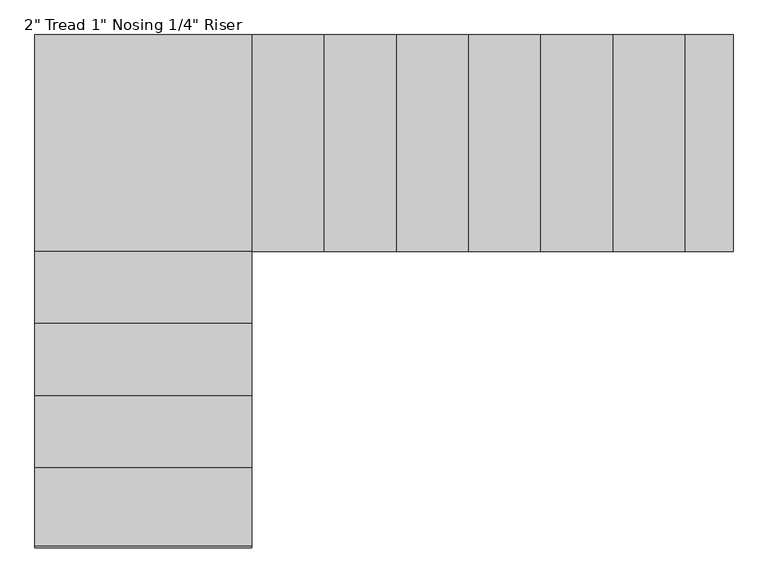
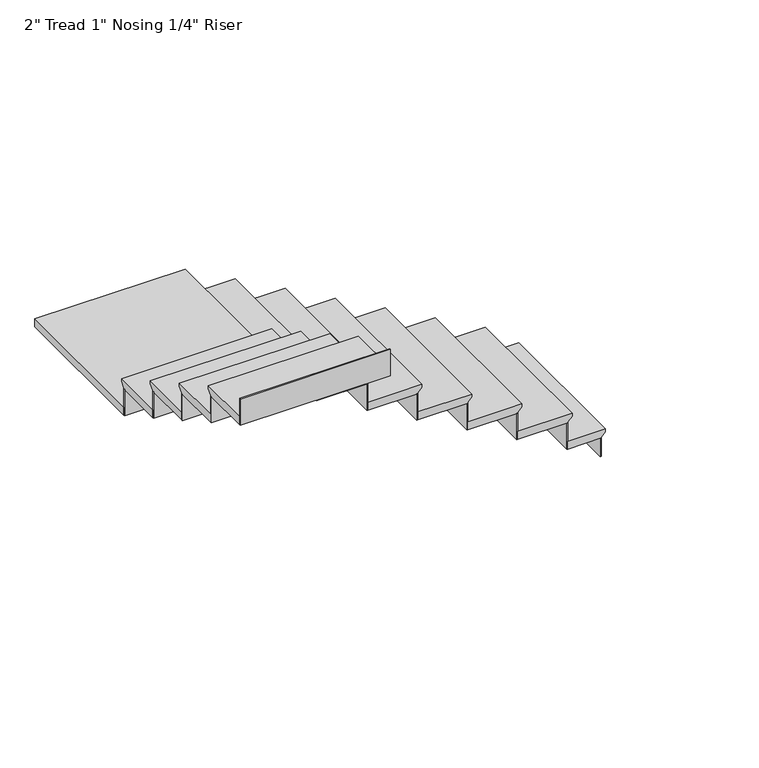
"""IFC4 building model written with IfcOpenShell, lengths in millimetres: stair flight geometry."""

from ifc_helpers import new_model, si_unit, origin, place, context, project, spatial, faceted_brep, source, transform, mapped, element, save


def stair_flight_cf719367(model_context):
    return source(origin(), model_context, "Body", "Brep", [
        faceted_brep([(-442.4415084, 5282.3381995, 3198.2833333), (-442.4415084, 5282.3381995, 3217.3333333), (-442.4415084, 4368.3146777, 3217.3333333), (-442.4415084, 4368.3146777, 3198.2833333), (-467.8415084, 5282.3381995, 3172.8833333), (-467.8415084, 4368.3146777, 3172.8833333), (-671.0415084, 5282.3381995, 3217.3333333), (-671.0415084, 4368.3146777, 3217.3333333), (-467.8415084, 4368.3146777, 3166.5333333), (-671.0415084, 4368.3146777, 3166.5333333), (-671.0415084, 5282.3381995, 3166.5333333), (-467.8415084, 5282.3381995, 3166.5333333)], [[[0, 1, 2, 3]], [[4, 0, 3, 5]], [[2, 1, 6, 7]], [[8, 9, 10, 11]], [[2, 7, 9, 8, 5, 3]], [[8, 11, 4, 5]], [[6, 1, 0, 4, 11, 10]], [[7, 6, 10, 9]]]),
        faceted_brep([(-467.8415084, 5282.3381995, 3166.5333333), (-467.8415084, 5282.3381995, 3048.0), (-474.1915084, 5282.3381995, 3048.0), (-474.1915084, 5282.3381995, 3166.5333333), (-467.8415084, 4368.3146777, 3166.5333333), (-474.1915084, 4368.3146777, 3166.5333333), (-474.1915084, 4368.3146777, 3048.0), (-467.8415084, 4368.3146777, 3048.0)], [[[0, 1, 2, 3]], [[4, 5, 6, 7]], [[1, 0, 4, 7]], [[2, 1, 7, 6]], [[3, 2, 6, 5]], [[0, 3, 5, 4]]]),
        faceted_brep([(-671.0415084, 5282.3381995, 3335.8666667), (-671.0415084, 5282.3381995, 3166.5333333), (-677.3915084, 5282.3381995, 3166.5333333), (-677.3915084, 5282.3381995, 3335.8666667), (-671.0415084, 4368.3146777, 3335.8666667), (-677.3915084, 4368.3146777, 3335.8666667), (-677.3915084, 4368.3146777, 3166.5333333), (-671.0415084, 4368.3146777, 3166.5333333)], [[[0, 1, 2, 3]], [[4, 5, 6, 7]], [[1, 0, 4, 7]], [[2, 1, 7, 6]], [[3, 2, 6, 5]], [[0, 3, 5, 4]]]),
        faceted_brep([(-645.6415084, 4368.3146777, 3386.6666667), (-645.6415084, 5282.3381995, 3386.6666667), (-975.8415084, 5282.3381995, 3386.6666667), (-975.8415084, 4368.3146777, 3386.6666667), (-671.0415084, 4368.3146777, 3335.8666667), (-975.8415084, 4368.3146777, 3335.8666667), (-975.8415084, 5282.3381995, 3335.8666667), (-671.0415084, 5282.3381995, 3335.8666667), (-671.0415084, 4368.3146777, 3342.2166667), (-645.6415084, 4368.3146777, 3367.6166667), (-671.0415084, 5282.3381995, 3342.2166667), (-645.6415084, 5282.3381995, 3367.6166667)], [[[0, 1, 2, 3]], [[4, 5, 6, 7]], [[0, 3, 5, 4, 8, 9]], [[4, 7, 10, 8]], [[2, 1, 11, 10, 7, 6]], [[3, 2, 6, 5]], [[11, 1, 0, 9]], [[10, 11, 9, 8]]]),
        faceted_brep([(-975.8415084, 5282.3381995, 3505.2), (-975.8415084, 5282.3381995, 3335.8666667), (-982.1915084, 5282.3381995, 3335.8666667), (-982.1915084, 5282.3381995, 3505.2), (-975.8415084, 4368.3146777, 3505.2), (-982.1915084, 4368.3146777, 3505.2), (-982.1915084, 4368.3146777, 3335.8666667), (-975.8415084, 4368.3146777, 3335.8666667)], [[[0, 1, 2, 3]], [[4, 5, 6, 7]], [[1, 0, 4, 7]], [[2, 1, 7, 6]], [[3, 2, 6, 5]], [[0, 3, 5, 4]]]),
        faceted_brep([(-950.4415084, 4368.3146777, 3556.0), (-950.4415084, 5282.3381995, 3556.0), (-1280.6415084, 5282.3381995, 3556.0), (-1280.6415084, 4368.3146777, 3556.0), (-975.8415084, 4368.3146777, 3505.2), (-1280.6415084, 4368.3146777, 3505.2), (-1280.6415084, 5282.3381995, 3505.2), (-975.8415084, 5282.3381995, 3505.2), (-975.8415084, 4368.3146777, 3511.55), (-950.4415084, 4368.3146777, 3536.95), (-975.8415084, 5282.3381995, 3511.55), (-950.4415084, 5282.3381995, 3536.95)], [[[0, 1, 2, 3]], [[4, 5, 6, 7]], [[0, 3, 5, 4, 8, 9]], [[4, 7, 10, 8]], [[2, 1, 11, 10, 7, 6]], [[3, 2, 6, 5]], [[11, 1, 0, 9]], [[10, 11, 9, 8]]]),
        faceted_brep([(-1280.6415084, 5282.3381995, 3674.5333333), (-1280.6415084, 5282.3381995, 3505.2), (-1286.9915084, 5282.3381995, 3505.2), (-1286.9915084, 5282.3381995, 3674.5333333), (-1280.6415084, 4368.3146777, 3674.5333333), (-1286.9915084, 4368.3146777, 3674.5333333), (-1286.9915084, 4368.3146777, 3505.2), (-1280.6415084, 4368.3146777, 3505.2)], [[[0, 1, 2, 3]], [[4, 5, 6, 7]], [[1, 0, 4, 7]], [[2, 1, 7, 6]], [[3, 2, 6, 5]], [[0, 3, 5, 4]]]),
        faceted_brep([(-1255.2415084, 4368.3146777, 3725.3333333), (-1255.2415084, 5282.3381995, 3725.3333333), (-1585.4415084, 5282.3381995, 3725.3333333), (-1585.4415084, 4368.3146777, 3725.3333333), (-1280.6415084, 4368.3146777, 3674.5333333), (-1585.4415084, 4368.3146777, 3674.5333333), (-1585.4415084, 5282.3381995, 3674.5333333), (-1280.6415084, 5282.3381995, 3674.5333333), (-1280.6415084, 4368.3146777, 3680.8833333), (-1255.2415084, 4368.3146777, 3706.2833333), (-1280.6415084, 5282.3381995, 3680.8833333), (-1255.2415084, 5282.3381995, 3706.2833333)], [[[0, 1, 2, 3]], [[4, 5, 6, 7]], [[0, 3, 5, 4, 8, 9]], [[4, 7, 10, 8]], [[2, 1, 11, 10, 7, 6]], [[3, 2, 6, 5]], [[11, 1, 0, 9]], [[10, 11, 9, 8]]]),
        faceted_brep([(-1585.4415084, 5282.3381995, 3843.8666667), (-1585.4415084, 5282.3381995, 3674.5333333), (-1591.7915084, 5282.3381995, 3674.5333333), (-1591.7915084, 5282.3381995, 3843.8666667), (-1585.4415084, 4368.3146777, 3843.8666667), (-1591.7915084, 4368.3146777, 3843.8666667), (-1591.7915084, 4368.3146777, 3674.5333333), (-1585.4415084, 4368.3146777, 3674.5333333)], [[[0, 1, 2, 3]], [[4, 5, 6, 7]], [[1, 0, 4, 7]], [[2, 1, 7, 6]], [[3, 2, 6, 5]], [[0, 3, 5, 4]]]),
        faceted_brep([(-1560.0415084, 4368.3146777, 3894.6666667), (-1560.0415084, 5282.3381995, 3894.6666667), (-1890.2415084, 5282.3381995, 3894.6666667), (-1890.2415084, 4368.3146777, 3894.6666667), (-1585.4415084, 4368.3146777, 3843.8666667), (-1890.2415084, 4368.3146777, 3843.8666667), (-1890.2415084, 5282.3381995, 3843.8666667), (-1585.4415084, 5282.3381995, 3843.8666667), (-1585.4415084, 4368.3146777, 3850.2166667), (-1560.0415084, 4368.3146777, 3875.6166667), (-1585.4415084, 5282.3381995, 3850.2166667), (-1560.0415084, 5282.3381995, 3875.6166667)], [[[0, 1, 2, 3]], [[4, 5, 6, 7]], [[0, 3, 5, 4, 8, 9]], [[4, 7, 10, 8]], [[2, 1, 11, 10, 7, 6]], [[3, 2, 6, 5]], [[11, 1, 0, 9]], [[10, 11, 9, 8]]]),
        faceted_brep([(-1890.2415084, 5282.3381995, 4013.2), (-1890.2415084, 5282.3381995, 3843.8666667), (-1896.5915084, 5282.3381995, 3843.8666667), (-1896.5915084, 5282.3381995, 4013.2), (-1890.2415084, 4368.3146777, 4013.2), (-1896.5915084, 4368.3146777, 4013.2), (-1896.5915084, 4368.3146777, 3843.8666667), (-1890.2415084, 4368.3146777, 3843.8666667)], [[[0, 1, 2, 3]], [[4, 5, 6, 7]], [[1, 0, 4, 7]], [[2, 1, 7, 6]], [[3, 2, 6, 5]], [[0, 3, 5, 4]]]),
        faceted_brep([(-1864.8415084, 4368.3146777, 4064.0), (-1864.8415084, 5282.3381995, 4064.0), (-2195.0415084, 5282.3381995, 4064.0), (-2195.0415084, 4368.3146777, 4064.0), (-1890.2415084, 4368.3146777, 4013.2), (-2195.0415084, 4368.3146777, 4013.2), (-2195.0415084, 5282.3381995, 4013.2), (-1890.2415084, 5282.3381995, 4013.2), (-1890.2415084, 4368.3146777, 4019.55), (-1864.8415084, 4368.3146777, 4044.95), (-1890.2415084, 5282.3381995, 4019.55), (-1864.8415084, 5282.3381995, 4044.95)], [[[0, 1, 2, 3]], [[4, 5, 6, 7]], [[0, 3, 5, 4, 8, 9]], [[4, 7, 10, 8]], [[2, 1, 11, 10, 7, 6]], [[3, 2, 6, 5]], [[11, 1, 0, 9]], [[10, 11, 9, 8]]]),
        faceted_brep([(-2195.0415084, 5282.3381995, 4182.5333333), (-2195.0415084, 5282.3381995, 4013.2), (-2201.3915084, 5282.3381995, 4013.2), (-2201.3915084, 5282.3381995, 4182.5333333), (-2195.0415084, 4368.3146777, 4182.5333333), (-2201.3915084, 4368.3146777, 4182.5333333), (-2201.3915084, 4368.3146777, 4013.2), (-2195.0415084, 4368.3146777, 4013.2)], [[[0, 1, 2, 3]], [[4, 5, 6, 7]], [[1, 0, 4, 7]], [[2, 1, 7, 6]], [[3, 2, 6, 5]], [[0, 3, 5, 4]]]),
        faceted_brep([(-2169.6415084, 4368.3146777, 4233.3333333), (-2169.6415084, 5282.3381995, 4233.3333333), (-2499.8415084, 5282.3381995, 4233.3333333), (-2499.8415084, 4368.3146777, 4233.3333333), (-2195.0415084, 4368.3146777, 4182.5333333), (-2499.8415084, 4368.3146777, 4182.5333333), (-2499.8415084, 5282.3381995, 4182.5333333), (-2195.0415084, 5282.3381995, 4182.5333333), (-2195.0415084, 4368.3146777, 4188.8833333), (-2169.6415084, 4368.3146777, 4214.2833333), (-2195.0415084, 5282.3381995, 4188.8833333), (-2169.6415084, 5282.3381995, 4214.2833333)], [[[0, 1, 2, 3]], [[4, 5, 6, 7]], [[0, 3, 5, 4, 8, 9]], [[4, 7, 10, 8]], [[2, 1, 11, 10, 7, 6]], [[3, 2, 6, 5]], [[11, 1, 0, 9]], [[10, 11, 9, 8]]]),
        faceted_brep([(-2499.8415084, 5282.3381995, 4351.8666667), (-2499.8415084, 5282.3381995, 4182.5333333), (-2506.1915084, 5282.3381995, 4182.5333333), (-2506.1915084, 5282.3381995, 4351.8666667), (-2499.8415084, 4368.3146777, 4351.8666667), (-2506.1915084, 4368.3146777, 4351.8666667), (-2506.1915084, 4368.3146777, 4182.5333333), (-2499.8415084, 4368.3146777, 4182.5333333)], [[[0, 1, 2, 3]], [[4, 5, 6, 7]], [[1, 0, 4, 7]], [[2, 1, 7, 6]], [[3, 2, 6, 5]], [[0, 3, 5, 4]]]),
        faceted_brep([(-3388.8415084, 5282.3381995, 4402.6666667), (-3388.8415084, 4342.9146777, 4402.6666667), (-2474.4415084, 4342.9146777, 4402.6666667), (-2474.4415084, 5282.3381995, 4402.6666667), (-2474.4415084, 4368.3146777, 4351.8666667), (-2474.4415084, 4342.9146777, 4351.8666667), (-3388.8415084, 4342.9146777, 4351.8666667), (-3388.8415084, 5282.3381995, 4351.8666667), (-2499.8415084, 5282.3381995, 4351.8666667), (-2499.8415084, 4368.3146777, 4351.8666667), (-2474.4415084, 4368.3146777, 4383.6166667), (-2474.4415084, 5282.3381995, 4383.6166667), (-2499.8415084, 4368.3146777, 4358.2166667), (-2499.8415084, 5282.3381995, 4358.2166667)], [[[0, 1, 2, 3]], [[4, 5, 6, 7, 8, 9]], [[3, 2, 5, 4, 10, 11]], [[4, 9, 12, 10]], [[9, 8, 13, 12]], [[0, 3, 11, 13, 8, 7]], [[1, 0, 7, 6]], [[2, 1, 6, 5]], [[13, 11, 10, 12]]]),
        faceted_brep([(-3388.8415084, 4342.9146777, 4521.2), (-3388.8415084, 4342.9146777, 4351.8666667), (-3388.8415084, 4336.5646777, 4351.8666667), (-3388.8415084, 4336.5646777, 4521.2), (-2474.4415084, 4342.9146777, 4521.2), (-2474.4415084, 4336.5646777, 4521.2), (-2474.4415084, 4336.5646777, 4351.8666667), (-2474.4415084, 4342.9146777, 4351.8666667)], [[[0, 1, 2, 3]], [[4, 5, 6, 7]], [[1, 0, 4, 7]], [[2, 1, 7, 6]], [[3, 2, 6, 5]], [[0, 3, 5, 4]]]),
        faceted_brep([(-2474.4415084, 4368.3146777, 4572.0), (-3388.8415084, 4368.3146777, 4572.0), (-3388.8415084, 4037.7382512, 4572.0), (-2474.4415084, 4037.7382512, 4572.0), (-2474.4415084, 4342.9146777, 4521.2), (-2474.4415084, 4037.7382512, 4521.2), (-3388.8415084, 4037.7382512, 4521.2), (-3388.8415084, 4342.9146777, 4521.2), (-2474.4415084, 4342.9146777, 4527.55), (-2474.4415084, 4368.3146777, 4552.95), (-3388.8415084, 4342.9146777, 4527.55), (-3388.8415084, 4368.3146777, 4552.95)], [[[0, 1, 2, 3]], [[4, 5, 6, 7]], [[0, 3, 5, 4, 8, 9]], [[4, 7, 10, 8]], [[2, 1, 11, 10, 7, 6]], [[3, 2, 6, 5]], [[11, 1, 0, 9]], [[10, 11, 9, 8]]]),
        faceted_brep([(-3388.8415084, 4037.7382512, 4690.5333333), (-3388.8415084, 4037.7382512, 4521.2), (-3388.8415084, 4031.3882512, 4521.2), (-3388.8415084, 4031.3882512, 4690.5333333), (-2474.4415084, 4037.7382512, 4690.5333333), (-2474.4415084, 4031.3882512, 4690.5333333), (-2474.4415084, 4031.3882512, 4521.2), (-2474.4415084, 4037.7382512, 4521.2)], [[[0, 1, 2, 3]], [[4, 5, 6, 7]], [[1, 0, 4, 7]], [[2, 1, 7, 6]], [[3, 2, 6, 5]], [[0, 3, 5, 4]]]),
        faceted_brep([(-2474.4415084, 4063.1382512, 4741.3333333), (-3388.8415084, 4063.1382512, 4741.3333333), (-3388.8415084, 3732.938277, 4741.3333333), (-2474.4415084, 3732.938277, 4741.3333333), (-2474.4415084, 4037.7382512, 4690.5333333), (-2474.4415084, 3732.938277, 4690.5333333), (-3388.8415084, 3732.938277, 4690.5333333), (-3388.8415084, 4037.7382512, 4690.5333333), (-2474.4415084, 4037.7382512, 4696.8833333), (-2474.4415084, 4063.1382512, 4722.2833333), (-3388.8415084, 4037.7382512, 4696.8833333), (-3388.8415084, 4063.1382512, 4722.2833333)], [[[0, 1, 2, 3]], [[4, 5, 6, 7]], [[0, 3, 5, 4, 8, 9]], [[4, 7, 10, 8]], [[2, 1, 11, 10, 7, 6]], [[3, 2, 6, 5]], [[11, 1, 0, 9]], [[10, 11, 9, 8]]]),
        faceted_brep([(-3388.8415084, 3732.938277, 4859.8666667), (-3388.8415084, 3732.938277, 4690.5333333), (-3388.8415084, 3726.588277, 4690.5333333), (-3388.8415084, 3726.588277, 4859.8666667), (-2474.4415084, 3732.938277, 4859.8666667), (-2474.4415084, 3726.588277, 4859.8666667), (-2474.4415084, 3726.588277, 4690.5333333), (-2474.4415084, 3732.938277, 4690.5333333)], [[[0, 1, 2, 3]], [[4, 5, 6, 7]], [[1, 0, 4, 7]], [[2, 1, 7, 6]], [[3, 2, 6, 5]], [[0, 3, 5, 4]]]),
        faceted_brep([(-2474.4415084, 3758.338277, 4910.6666667), (-3388.8415084, 3758.338277, 4910.6666667), (-3388.8415084, 3428.1383028, 4910.6666667), (-2474.4415084, 3428.1383028, 4910.6666667), (-2474.4415084, 3732.938277, 4859.8666667), (-2474.4415084, 3428.1383028, 4859.8666667), (-3388.8415084, 3428.1383028, 4859.8666667), (-3388.8415084, 3732.938277, 4859.8666667), (-2474.4415084, 3732.938277, 4866.2166667), (-2474.4415084, 3758.338277, 4891.6166667), (-3388.8415084, 3732.938277, 4866.2166667), (-3388.8415084, 3758.338277, 4891.6166667)], [[[0, 1, 2, 3]], [[4, 5, 6, 7]], [[0, 3, 5, 4, 8, 9]], [[4, 7, 10, 8]], [[2, 1, 11, 10, 7, 6]], [[3, 2, 6, 5]], [[11, 1, 0, 9]], [[10, 11, 9, 8]]]),
        faceted_brep([(-3388.8415084, 3428.1383028, 5029.2), (-3388.8415084, 3428.1383028, 4859.8666667), (-3388.8415084, 3421.7883028, 4859.8666667), (-3388.8415084, 3421.7883028, 5029.2), (-2474.4415084, 3428.1383028, 5029.2), (-2474.4415084, 3421.7883028, 5029.2), (-2474.4415084, 3421.7883028, 4859.8666667), (-2474.4415084, 3428.1383028, 4859.8666667)], [[[0, 1, 2, 3]], [[4, 5, 6, 7]], [[1, 0, 4, 7]], [[2, 1, 7, 6]], [[3, 2, 6, 5]], [[0, 3, 5, 4]]]),
        faceted_brep([(-3388.8415084, 3123.3383287, 5198.5333333), (-3388.8415084, 3123.3383287, 5029.2), (-3388.8415084, 3116.9883287, 5029.2), (-3388.8415084, 3116.9883287, 5198.5333333), (-2474.4415084, 3123.3383287, 5198.5333333), (-2474.4415084, 3116.9883287, 5198.5333333), (-2474.4415084, 3116.9883287, 5029.2), (-2474.4415084, 3123.3383287, 5029.2)], [[[0, 1, 2, 3]], [[4, 5, 6, 7]], [[1, 0, 4, 7]], [[2, 1, 7, 6]], [[3, 2, 6, 5]], [[0, 3, 5, 4]]]),
        faceted_brep([(-2474.4415084, 3453.5383028, 5080.0), (-3388.8415084, 3453.5383028, 5080.0), (-3388.8415084, 3123.3383287, 5080.0), (-2474.4415084, 3123.3383287, 5080.0), (-2474.4415084, 3428.1383028, 5029.2), (-2474.4415084, 3123.3383287, 5029.2), (-3388.8415084, 3123.3383287, 5029.2), (-3388.8415084, 3428.1383028, 5029.2), (-2474.4415084, 3428.1383028, 5035.55), (-2474.4415084, 3453.5383028, 5060.95), (-3388.8415084, 3428.1383028, 5035.55), (-3388.8415084, 3453.5383028, 5060.95)], [[[0, 1, 2, 3]], [[4, 5, 6, 7]], [[0, 3, 5, 4, 8, 9]], [[4, 7, 10, 8]], [[2, 1, 11, 10, 7, 6]], [[3, 2, 6, 5]], [[11, 1, 0, 9]], [[10, 11, 9, 8]]]),
    ])


if __name__ == "__main__":
    model = new_model("IFC4")
    model_context = context("Model", 3, world=origin())
    ifc_project = project(units=[si_unit("LENGTHUNIT", "METRE", prefix="MILLI")], contexts=[model_context])
    site = spatial("IfcSite", under=ifc_project)
    building = spatial("IfcBuilding", under=site)
    placement = place(None, origin())
    stair_flight_shape = stair_flight_cf719367(model_context)
    element("IfcStairFlight", 1, ObjectType="2\" Tread 1\" Nosing 1/4\" Riser", at=placement, inside=building, context=model_context, shape_type="MappedRepresentation", body=[
        mapped(stair_flight_shape, transform((0.0, 0.0, 0.0), x_axis=(1.0, 0.0, 0.0), y_axis=(0.0, 1.0, 0.0), z_axis=(0.0, 0.0, 1.0))),
    ])
    save(model, "model.ifc")
